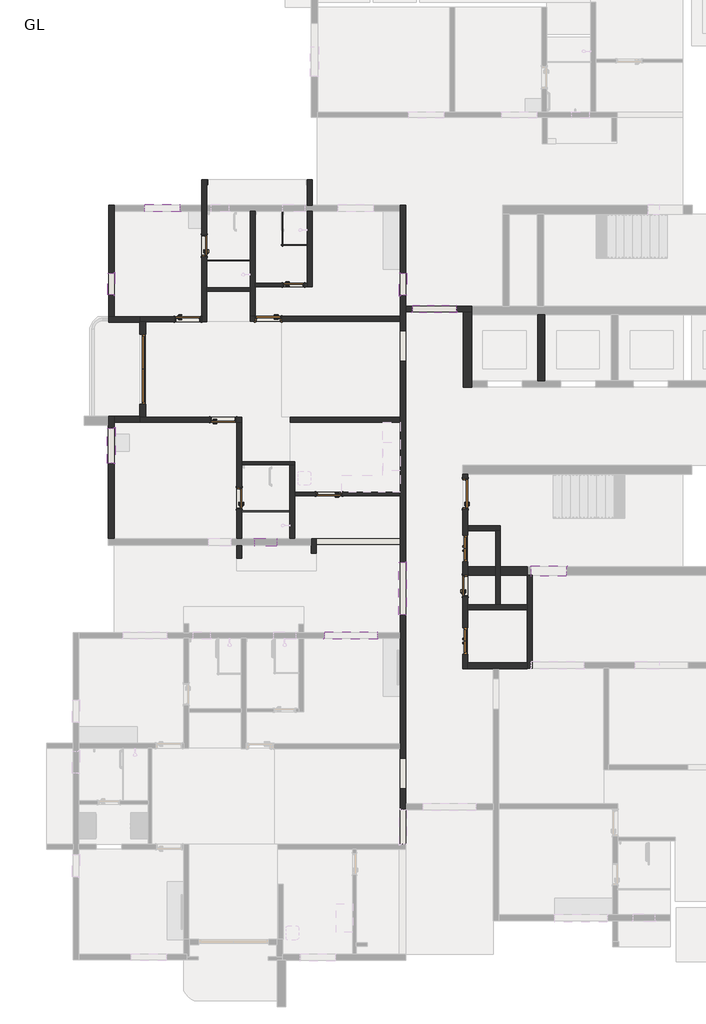
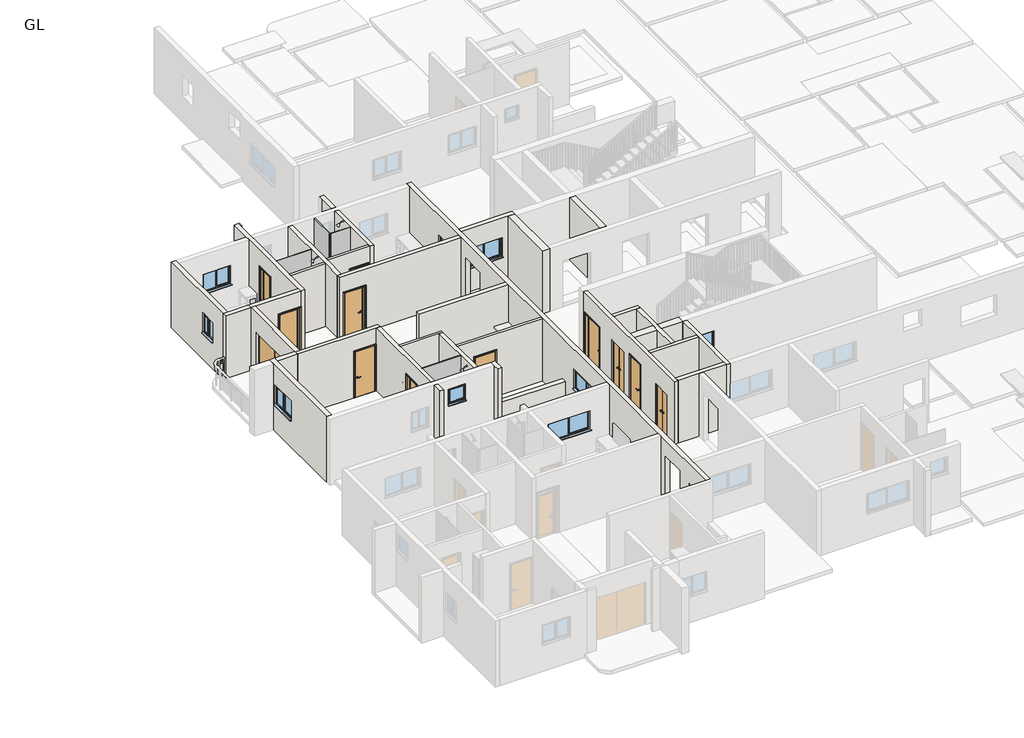
# One storey, part 2 of 14: 32 walls, 12 doors, 9 windows, 4 plates.
"""IFC4 building model written with IfcOpenShell, lengths in millimetres."""

from ifc_helpers import new_model, si_unit, frame, origin, origin_with_axes, place, context, project, spatial, polyline, outline, extrude, faceted_brep, transform, mapped, element, save
from components import doors_concept_extdbl_8_c180431f, doors_extdbl_flush_3_6b548a76, doors_intsgl_2_5_door_21b53886, doors_intsgl_2_5_door_57e365e7, doors_intsgl_2_5_door_fd097d29, doors_intsgl_2_5_door_b929695a, doors_intsgl_3_door_8261d8fb, doors_intsgl_3_door_f61d7fb9, doors_intsgl_3_door_77e94e6e, doors_intsgl_3_door_2f660dd7, doors_intsgl_3_5_a4e1cc10, system_panel_glazed_00f127ae, system_panel_glazed_4e689a8f, system_panel_glazed_de536e8c, system_panel_glazed_7a5adaf1, windows_dbl_plain_2_5_52f1e8c5, windows_dbl_plain_4_e08ba9e4, windows_dbl_plain_4_905afcad, windows_dbl_plain_4_ad201dc9, windows_dbl_plain_5_c7724a63, windows_dbl_plain_6_decf5736, windows_sgl_plain_2_5_1233c963

model = new_model("IFC4")

# Units and contexts
model_context = context("Model", 3, world=origin())
ifc_project = project(units=[si_unit("LENGTHUNIT", "METRE", prefix="MILLI")], contexts=[model_context])

# Site, building, storey
site = spatial("IfcSite", under=ifc_project)
building = spatial("IfcBuilding", under=site)
storey = spatial("IfcBuildingStorey", under=building, Name="GL", Elevation=0.0)

# Doors
placement = place(None, origin())
doors_concept_extdbl_8_shape = doors_concept_extdbl_8_c180431f(model_context)
element("IfcDoor", 1, ObjectType="Doors_Concept_ExtDbl : 8'", at=placement, inside=storey, context=model_context, shape_type="MappedRepresentation", body=[
    mapped(doors_concept_extdbl_8_shape, transform((-14465.3631346, 76757.5607361, 0.0), x_axis=(0.0, -1.0, 0.0), y_axis=(1.0, 0.0, 0.0), z_axis=(0.0, 0.0, 1.0))),
])
doors_extdbl_flush_3_shape = doors_extdbl_flush_3_6b548a76(model_context)
element("IfcDoor", 2, ObjectType="Doors_ExtDbl_Flush : 3'", at=placement, inside=storey, context=model_context, shape_type="MappedRepresentation", body=[
    mapped(doors_extdbl_flush_3_shape, transform((-3221.1847841, 67274.0128421, 0.0), x_axis=(0.0, -1.0, 0.0), y_axis=(1.0, 0.0, 0.0), z_axis=(0.0, 0.0, 1.0))),
])
element("IfcDoor", 3, ObjectType="Doors_ExtDbl_Flush : 3'", at=placement, inside=storey, context=model_context, shape_type="MappedRepresentation", body=[
    mapped(doors_extdbl_flush_3_shape, transform((-3221.1847841, 70498.5428421, 0.0), x_axis=(0.0, -1.0, 0.0), y_axis=(1.0, 0.0, 0.0), z_axis=(0.0, 0.0, 1.0))),
])
doors_intsgl_2_5_door_shape = doors_intsgl_2_5_door_21b53886(model_context)
element("IfcDoor", 4, ObjectType="Doors_IntSgl : 2.5' DOOR", at=placement, inside=storey, context=model_context, shape_type="MappedRepresentation", body=[
    mapped(doors_intsgl_2_5_door_shape, transform((-9206.9991708, 79690.7146999, 149.9616), x_axis=(1.0, 0.0, 0.0), y_axis=(0.0, 1.0, 0.0), z_axis=(0.0, 0.0, 1.0))),
])
doors_intsgl_2_5_door_2_shape = doors_intsgl_2_5_door_57e365e7(model_context)
element("IfcDoor", 5, ObjectType="Doors_IntSgl : 2.5' DOOR", at=placement, inside=storey, context=model_context, shape_type="MappedRepresentation", body=[
    mapped(doors_intsgl_2_5_door_2_shape, transform((-11094.7831346, 72249.3527724, 149.9616), x_axis=(0.0, 1.0, 0.0), y_axis=(-1.0, 0.0, 0.0), z_axis=(0.0, 0.0, 1.0))),
])
doors_intsgl_2_5_door_3_shape = doors_intsgl_2_5_door_fd097d29(model_context)
element("IfcDoor", 6, ObjectType="Doors_IntSgl : 2.5' DOOR", at=placement, inside=storey, context=model_context, shape_type="MappedRepresentation", body=[
    mapped(doors_intsgl_2_5_door_3_shape, transform((-12321.0850072, 81060.5334496, 149.9616), x_axis=(0.0, 1.0, 0.0), y_axis=(-1.0, 0.0, 0.0), z_axis=(0.0, 0.0, 1.0))),
])
doors_intsgl_2_5_door_4_shape = doors_intsgl_2_5_door_b929695a(model_context)
element("IfcDoor", 7, ObjectType="Doors_IntSgl : 2.5' DOOR", at=placement, inside=storey, context=model_context, shape_type="MappedRepresentation", body=[
    mapped(doors_intsgl_2_5_door_4_shape, transform((-3221.1847841, 69198.0628421, 149.9616), x_axis=(0.0, 1.0, 0.0), y_axis=(-1.0, 0.0, 0.0), z_axis=(0.0, 0.0, 1.0))),
])
doors_intsgl_3_door_shape = doors_intsgl_3_door_8261d8fb(model_context)
element("IfcDoor", 8, ObjectType="Doors_IntSgl : 3' DOOR", at=placement, inside=storey, context=model_context, shape_type="MappedRepresentation", body=[
    mapped(doors_intsgl_3_door_shape, transform((-10090.2131346, 78505.8807724, 149.9616), x_axis=(-1.0, 0.0, 0.0), y_axis=(0.0, -1.0, 0.0), z_axis=(0.0, 0.0, 1.0))),
])
doors_intsgl_3_door_2_shape = doors_intsgl_3_door_f61d7fb9(model_context)
element("IfcDoor", 9, ObjectType="Doors_IntSgl : 3' DOOR", at=placement, inside=storey, context=model_context, shape_type="MappedRepresentation", body=[
    mapped(doors_intsgl_3_door_2_shape, transform((-12890.5530072, 78496.4066999, 149.9616), x_axis=(1.0, 0.0, 0.0), y_axis=(0.0, 1.0, 0.0), z_axis=(0.0, 0.0, 1.0))),
])
doors_intsgl_3_door_3_shape = doors_intsgl_3_door_77e94e6e(model_context)
element("IfcDoor", 10, ObjectType="Doors_IntSgl : 3' DOOR", at=placement, inside=storey, context=model_context, shape_type="MappedRepresentation", body=[
    mapped(doors_intsgl_3_door_3_shape, transform((-7969.3131346, 72401.7527724, 149.9616), x_axis=(-1.0, 0.0, 0.0), y_axis=(0.0, -1.0, 0.0), z_axis=(0.0, 0.0, 1.0))),
])
doors_intsgl_3_door_4_shape = doors_intsgl_3_door_2f660dd7(model_context)
element("IfcDoor", 11, ObjectType="Doors_IntSgl : 3' DOOR", at=placement, inside=storey, context=model_context, shape_type="MappedRepresentation", body=[
    mapped(doors_intsgl_3_door_4_shape, transform((-11661.2031346, 74991.2827724, 149.9616), x_axis=(1.0, 0.0, 0.0), y_axis=(0.0, 1.0, 0.0), z_axis=(0.0, 0.0, 1.0))),
])
doors_intsgl_3_5_shape = doors_intsgl_3_5_a4e1cc10(model_context)
element("IfcDoor", 12, ObjectType="Doors_IntSgl : 3.5'", at=placement, inside=storey, context=model_context, shape_type="MappedRepresentation", body=[
    mapped(doors_intsgl_3_5_shape, transform((-3221.1847841, 72409.8178911, 0.0), x_axis=(0.0, 1.0, 0.0), y_axis=(-1.0, 0.0, 0.0), z_axis=(0.0, 0.0, 1.0))),
])

# Plates
system_panel_glazed_shape = system_panel_glazed_00f127ae(model_context)
element("IfcPlate", 13, ObjectType="System Panel : Glazed", at=placement, inside=storey, context=model_context, shape_type="MappedRepresentation", body=[
    mapped(system_panel_glazed_shape, transform((-9632.2131346, 81643.1046999, 0.0), x_axis=(0.0, -1.0, 0.0), y_axis=(1.0, 0.0, 0.0), z_axis=(0.0, 0.0, 1.0))),
])
system_panel_glazed_2_shape = system_panel_glazed_4e689a8f(model_context)
element("IfcPlate", 14, ObjectType="System Panel : Glazed", at=placement, inside=storey, context=model_context, shape_type="MappedRepresentation", body=[
    mapped(system_panel_glazed_2_shape, transform((-10179.437141, 71760.4027724, 0.0), x_axis=(1.0, 0.0, 0.0), y_axis=(0.0, 1.0, 0.0), z_axis=(0.0, 0.0, 1.0))),
])
system_panel_glazed_3_shape = system_panel_glazed_de536e8c(model_context)
element("IfcPlate", 15, ObjectType="System Panel : Glazed", at=placement, inside=storey, context=model_context, shape_type="MappedRepresentation", body=[
    mapped(system_panel_glazed_3_shape, transform((-11477.6830709, 80509.8646999, 0.0), x_axis=(1.0, 0.0, 0.0), y_axis=(0.0, 1.0, 0.0), z_axis=(0.0, 0.0, 1.0))),
])
system_panel_glazed_4_shape = system_panel_glazed_7a5adaf1(model_context)
element("IfcPlate", 16, ObjectType="System Panel : Glazed", at=placement, inside=storey, context=model_context, shape_type="MappedRepresentation", body=[
    mapped(system_panel_glazed_4_shape, transform((-9178.3061527, 81046.2046999, 0.0), x_axis=(1.0, 0.0, 0.0), y_axis=(0.0, 1.0, 0.0), z_axis=(0.0, 0.0, 1.0))),
])

# Walls
element("IfcWall", 17, ObjectType="W2", at=placement, inside=storey, context=model_context, shape_type="SweptSolid", body=[
    extrude(outline(polyline([(-9328.2131346, 75074.8487724), (-5492.8131346, 75074.8487724), (-5492.8131346, 74901.1127724), (-9328.2131346, 74901.1127724), (-9328.2131346, 75074.8487724)])), origin_with_axes(), (0.0, 0.0, 1.0), 3000.0),
])
element("IfcWall", 18, ObjectType="W2", at=placement, inside=storey, context=model_context, shape_type="Brep", body=[
    faceted_brep([(-5492.8131346, 78592.7487724, 0.0), (-10547.4131346, 78592.7487724, 0.0), (-10721.1491346, 78592.7487724, 0.0), (-10721.1491346, 78592.7487724, 3000.0), (-10547.4131346, 78592.7487724, 3000.0), (-5492.8131346, 78592.7487724, 3000.0), (-10547.4131346, 78592.7487724, 2259.9616), (-10547.4131346, 78592.7487724, 149.9616), (-9633.0131346, 78592.7487724, 149.9616), (-9633.0131346, 78592.7487724, 2259.9616), (-10721.1491346, 78419.0127724, 0.0), (-5492.8131346, 78419.0127724, 0.0), (-5492.8131346, 78419.0127724, 3000.0), (-10721.1491346, 78419.0127724, 3000.0), (-10547.4131346, 78419.0127724, 149.9616), (-10547.4131346, 78419.0127724, 2259.9616), (-9633.0131346, 78419.0127724, 2259.9616), (-9633.0131346, 78419.0127724, 149.9616)], [[[0, 1, 2, 3, 4, 5], [6, 7, 8, 9]], [[10, 11, 12, 13], [14, 15, 16, 17]], [[2, 1, 0, 11, 10]], [[5, 4, 3, 13, 12]], [[0, 5, 12, 11]], [[3, 2, 10, 13]], [[14, 7, 6, 15]], [[15, 6, 9, 16]], [[16, 9, 8, 17]], [[7, 14, 17, 8]]]),
])
element("IfcWall", 19, ObjectType="W2", at=placement, inside=storey, context=model_context, shape_type="Brep", body=[
    faceted_brep([(-10547.4131346, 78592.7487724, 0.0), (-10547.4131346, 79633.5646999, 0.0), (-10547.4131346, 79747.8646999, 0.0), (-10547.4131346, 82265.0046999, 0.0), (-10547.4131346, 82265.0046999, 3000.0), (-10547.4131346, 79747.8646999, 3000.0), (-10547.4131346, 79633.5646999, 3000.0), (-10547.4131346, 78592.7487724, 3000.0), (-10547.4131346, 78592.7487724, 2110.0), (-10721.1491346, 78592.7487724, 0.0), (-10721.1491346, 78592.7487724, 3000.0), (-10721.1491346, 79473.0334496, 3000.0), (-10721.1491346, 79587.3334496, 3000.0), (-10721.1491346, 82265.0046999, 3000.0), (-10721.1491346, 82265.0046999, 0.0), (-10721.1491346, 79587.3334496, 0.0), (-10721.1491346, 79473.0334496, 0.0)], [[[0, 1, 2, 3, 4, 5, 6, 7, 8]], [[9, 10, 11, 12, 13, 14, 15, 16]], [[3, 2, 1, 0, 9, 16, 15, 14]], [[7, 6, 5, 4, 13, 12, 11, 10]], [[0, 8, 7, 10, 9]], [[4, 3, 14, 13]]]),
])
element("IfcWall", 20, ObjectType="W2", at=placement, inside=storey, context=model_context, shape_type="Brep", body=[
    faceted_brep([(-12234.2170072, 78409.5386999, 0.0), (-12234.2170072, 79473.0334496, 0.0), (-12234.2170072, 79587.3334496, 0.0), (-12234.2170072, 82265.0046999, 0.0), (-12234.2170072, 82463.1246999, 0.0), (-12234.2170072, 83194.026856, 0.0), (-12234.2170072, 83367.762856, 0.0), (-12234.2170072, 83367.762856, 3000.0), (-12234.2170072, 83194.026856, 3000.0), (-12234.2170072, 82463.1246999, 3000.0), (-12234.2170072, 82265.0046999, 3000.0), (-12234.2170072, 79587.3334496, 3000.0), (-12234.2170072, 79473.0334496, 3000.0), (-12234.2170072, 78409.5386999, 3000.0), (-12234.2170072, 81441.5334496, 2259.9616), (-12234.2170072, 81441.5334496, 149.9616), (-12234.2170072, 80679.5334496, 149.9616), (-12234.2170072, 80679.5334496, 2259.9616), (-12407.9530072, 83367.762856, 0.0), (-12407.9530072, 82463.1246999, 0.0), (-12407.9530072, 82265.0046999, 0.0), (-12407.9530072, 78583.2746999, 0.0), (-12407.9530072, 78409.5386999, 0.0), (-12407.9530072, 78409.5386999, 3000.0), (-12407.9530072, 78583.2746999, 3000.0), (-12407.9530072, 82265.0046999, 3000.0), (-12407.9530072, 82463.1246999, 3000.0), (-12407.9530072, 83367.762856, 3000.0), (-12407.9530072, 81441.5334496, 149.9616), (-12407.9530072, 81441.5334496, 2259.9616), (-12407.9530072, 80679.5334496, 2259.9616), (-12407.9530072, 80679.5334496, 149.9616)], [[[0, 1, 2, 3, 4, 5, 6, 7, 8, 9, 10, 11, 12, 13], [14, 15, 16, 17]], [[18, 19, 20, 21, 22, 23, 24, 25, 26, 27], [28, 29, 30, 31]], [[6, 5, 4, 3, 2, 1, 0, 22, 21, 20, 19, 18]], [[13, 12, 11, 10, 9, 8, 7, 27, 26, 25, 24, 23]], [[0, 13, 23, 22]], [[7, 6, 18, 27]], [[28, 15, 14, 29]], [[29, 14, 17, 30]], [[30, 17, 16, 31]], [[15, 28, 31, 16]]]),
])
element("IfcWall", 21, ObjectType="W2", at=placement, inside=storey, context=model_context, shape_type="Brep", body=[
    faceted_brep([(-12407.9530072, 78583.2746999, 0.0), (-14564.4231346, 78583.2746999, 0.0), (-14564.4231346, 78583.2746999, 3000.0), (-12407.9530072, 78583.2746999, 3000.0), (-12433.3530072, 78583.2746999, 149.9616), (-12433.3530072, 78583.2746999, 2259.9616), (-13347.7530072, 78583.2746999, 2259.9616), (-13347.7530072, 78583.2746999, 149.9616), (-14564.4231346, 78409.5386999, 0.0), (-14366.3031346, 78409.5386999, 0.0), (-12407.9530072, 78409.5386999, 0.0), (-12407.9530072, 78409.5386999, 3000.0), (-14366.3031346, 78409.5386999, 3000.0), (-14564.4231346, 78409.5386999, 3000.0), (-12433.3530072, 78409.5386999, 2259.9616), (-12433.3530072, 78409.5386999, 149.9616), (-13347.7530072, 78409.5386999, 149.9616), (-13347.7530072, 78409.5386999, 2259.9616)], [[[0, 1, 2, 3], [4, 5, 6, 7]], [[8, 9, 10, 11, 12, 13], [14, 15, 16, 17]], [[1, 0, 10, 9, 8]], [[3, 2, 13, 12, 11]], [[0, 3, 11, 10]], [[2, 1, 8, 13]], [[4, 15, 14, 5]], [[5, 14, 17, 6]], [[6, 17, 16, 7]], [[15, 4, 7, 16]]]),
])
element("IfcWall", 22, ObjectType="W2", at=placement, inside=storey, context=model_context, shape_type="Brep", body=[
    faceted_brep([(-9336.8491346, 73417.7527724, 0.0), (-9336.8491346, 70838.3827724, 0.0), (-9336.8491346, 70838.3827724, 3000.0), (-9336.8491346, 73417.7527724, 3000.0), (-9163.1131346, 73417.7527724, 0.0), (-9163.1131346, 73417.7527724, 3000.0), (-9163.1131346, 72458.9027724, 3000.0), (-9163.1131346, 72344.6027724, 3000.0), (-9163.1131346, 70838.3827724, 3000.0), (-9163.1131346, 70838.3827724, 0.0), (-9163.1131346, 72344.6027724, 0.0), (-9163.1131346, 72458.9027724, 0.0)], [[[0, 1, 2, 3]], [[4, 5, 6, 7, 8, 9, 10, 11]], [[1, 0, 4, 11, 10, 9]], [[3, 2, 8, 7, 6, 5]], [[0, 3, 5, 4]], [[2, 1, 9, 8]]]),
])
element("IfcWall", 23, ObjectType="W2", at=placement, inside=storey, context=model_context, shape_type="Brep", body=[
    faceted_brep([(-8724.3991708, 83367.762856, 3000.0), (-8724.3991708, 83367.762856, 0.0), (-8724.3991708, 83194.026856, 0.0), (-8724.3991708, 82463.1246999, 0.0), (-8724.3991708, 82463.1246999, 3000.0), (-8724.3991708, 83194.026856, 3000.0), (-8550.6631708, 83367.762856, 0.0), (-8550.6631708, 83367.762856, 3000.0), (-8550.6631708, 82463.1246999, 3000.0), (-8550.6631708, 82463.1246999, 0.0)], [[[0, 1, 2, 3, 4, 5]], [[6, 7, 8, 9]], [[1, 6, 9, 3, 2]], [[7, 0, 5, 4, 8]], [[4, 3, 9, 8]], [[1, 0, 7, 6]]]),
    faceted_brep([(-8724.3991708, 79633.5646999, 0.0), (-8724.3991708, 79633.5646999, 3000.0), (-8724.3991708, 79747.8646999, 3000.0), (-8724.3991708, 82265.0046999, 3000.0), (-8724.3991708, 82265.0046999, 0.0), (-8724.3991708, 79747.8646999, 0.0), (-8550.6631708, 79633.5646999, 3000.0), (-8550.6631708, 79633.5646999, 0.0), (-8550.6631708, 82265.0046999, 0.0), (-8550.6631708, 82265.0046999, 3000.0)], [[[0, 1, 2, 3, 4, 5]], [[6, 7, 8, 9]], [[7, 0, 5, 4, 8]], [[1, 6, 9, 3, 2]], [[4, 3, 9, 8]], [[1, 0, 7, 6]]]),
])
element("IfcWall", 24, ObjectType="W2", at=placement, inside=storey, context=model_context, shape_type="SweptSolid", body=[
    extrude(outline(polyline([(-12234.2170072, 83367.762856), (-12196.1170072, 83367.762856), (-12196.1170072, 83194.026856), (-12234.2170072, 83194.026856), (-12234.2170072, 83367.762856)])), origin_with_axes(), (0.0, 0.0, 1.0), 3000.0),
])
element("IfcWall", 25, ObjectType="W2", at=placement, inside=storey, context=model_context, shape_type="Brep", body=[
    faceted_brep([(-8587.5491346, 70838.3827724, 3000.0), (-8587.5491346, 70838.3827724, 0.0), (-8587.5491346, 70609.7827724, 0.0), (-8587.5491346, 70335.4627724, 0.0), (-8587.5491346, 70335.4627724, 3000.0), (-8587.5491346, 70609.7827724, 3000.0), (-8413.8131346, 70838.3827724, 0.0), (-8413.8131346, 70838.3827724, 1171.2), (-8413.8131346, 70838.3827724, 3000.0), (-8413.8131346, 70335.4627724, 3000.0), (-8413.8131346, 70335.4627724, 0.0), (-8413.8131346, 70640.2627724, 0.0)], [[[0, 1, 2, 3, 4, 5]], [[6, 7, 8, 9, 10, 11]], [[3, 2, 1, 6, 11, 10]], [[4, 3, 10, 9]], [[0, 5, 4, 9, 8]], [[0, 8, 7, 6, 1]]]),
])
element("IfcWall", 26, ObjectType="W3", at=placement, inside=storey, context=model_context, shape_type="Brep", body=[
    faceted_brep([(-11010.9631346, 73417.7527724, 0.0), (-9336.8491346, 73417.7527724, 0.0), (-9163.1131346, 73417.7527724, 0.0), (-9163.1131346, 73417.7527724, 3000.0), (-9336.8491346, 73417.7527724, 3000.0), (-11010.9631346, 73417.7527724, 3000.0), (-11010.9631346, 73532.0527724, 0.0), (-11010.9631346, 73532.0527724, 3000.0), (-9163.1131346, 73532.0527724, 3000.0), (-9163.1131346, 73532.0527724, 0.0)], [[[0, 1, 2, 3, 4, 5]], [[6, 7, 8, 9]], [[2, 1, 0, 6, 9]], [[5, 4, 3, 8, 7]], [[0, 5, 7, 6]], [[3, 2, 9, 8]]]),
])
element("IfcWall", 27, ObjectType="W3", at=placement, inside=storey, context=model_context, shape_type="SweptSolid", body=[
    extrude(outline(polyline([(0.0, -9163.1131346), (0.0, -5492.8131346), (3000.0, -5492.8131346), (3000.0, -9163.1131346), (0.0, -9163.1131346)]), holes=[polyline([(149.9616, -8426.5131346), (2259.9616, -8426.5131346), (2259.9616, -7512.1131346), (149.9616, -7512.1131346), (149.9616, -8426.5131346)])]), frame((0.0, 72344.6027724, 0.0), z_axis=(0.0, 1.0, 0.0), x_axis=(0.0, 0.0, 1.0)), (0.0, 0.0, 1.0), 114.3),
])
element("IfcWall", 28, ObjectType="W3", at=placement, inside=storey, context=model_context, shape_type="SweptSolid", body=[
    extrude(outline(polyline([(-10721.1491346, 79473.0334496), (-12234.2170072, 79473.0334496), (-12234.2170072, 79587.3334496), (-10721.1491346, 79587.3334496), (-10721.1491346, 79473.0334496)])), origin_with_axes(), (0.0, 0.0, 1.0), 3000.0),
])
element("IfcWall", 29, ObjectType="W3", at=placement, inside=storey, context=model_context, shape_type="SweptSolid", body=[
    extrude(outline(polyline([(0.0, -10547.4131346), (0.0, -8724.3991708), (3000.0, -8724.3991708), (3000.0, -10547.4131346), (0.0, -10547.4131346)]), holes=[polyline([(2259.9616, -8825.9991708), (149.9616, -8825.9991708), (149.9616, -9587.9991708), (2259.9616, -9587.9991708), (2259.9616, -8825.9991708)])]), frame((0.0, 79633.5646999, 0.0), z_axis=(0.0, 1.0, 0.0), x_axis=(0.0, 0.0, 1.0)), (0.0, 0.0, 1.0), 114.3),
])
element("IfcWall", 30, ObjectType="W4", at=placement, inside=storey, context=model_context, shape_type="Brep", body=[
    faceted_brep([(-3288.0931346, 78750.2287724, 0.0), (-3288.0931346, 76131.4887724, 0.0), (-3288.0931346, 76131.4887724, 3000.0), (-3288.0931346, 78750.2287724, 3000.0), (-2983.2931346, 78750.2287724, 0.0), (-2983.2931346, 78750.2287724, 3000.0), (-2983.2931346, 78643.5487724, 3000.0), (-2983.2931346, 76353.9927724, 3000.0), (-2983.2931346, 76131.4887724, 3000.0), (-2983.2931346, 76131.4887724, 0.0), (-2983.2931346, 76353.9927724, 0.0), (-2983.2931346, 78643.5487724, 0.0)], [[[0, 1, 2, 3]], [[4, 5, 6, 7, 8, 9, 10, 11]], [[1, 0, 4, 11, 10, 9]], [[3, 2, 8, 7, 6, 5]], [[0, 3, 5, 4]], [[2, 1, 9, 8]]]),
])
element("IfcWall", 31, ObjectType="W4", at=placement, inside=storey, context=model_context, shape_type="Brep", body=[
    faceted_brep([(-1053.026306, 69566.3628421, 0.0), (-1053.026306, 69566.3628421, 3000.0), (-1988.0147841, 69566.3628421, 3000.0), (-1988.0147841, 69566.3628421, 0.0), (-1053.026306, 69871.1628421, 3000.0), (-1053.026306, 69871.1628421, 0.0), (-1988.0147841, 69871.1628421, 0.0), (-1988.0147841, 69871.1628421, 3000.0), (-1053.026306, 69866.1033979, 0.0), (-1053.026306, 69866.1033979, 3000.0)], [[[0, 1, 2, 3]], [[4, 5, 6, 7]], [[5, 8, 0, 3, 6]], [[1, 9, 4, 7, 2]], [[1, 0, 8, 5, 4, 9]], [[3, 2, 7, 6]]]),
    faceted_brep([(-3137.3647841, 69566.3628421, 3000.0), (-3137.3647841, 69566.3628421, 0.0), (-2155.6547841, 69566.3628421, 0.0), (-2155.6547841, 69566.3628421, 3000.0), (-3137.3647841, 69871.1628421, 0.0), (-3137.3647841, 69871.1628421, 3000.0), (-2155.6547841, 69871.1628421, 3000.0), (-2155.6547841, 69871.1628421, 0.0)], [[[0, 1, 2, 3]], [[4, 5, 6, 7]], [[1, 4, 7, 2]], [[5, 0, 3, 6]], [[1, 0, 5, 4]], [[3, 2, 7, 6]]]),
])
element("IfcWall", 32, ObjectType="W6", at=placement, inside=storey, context=model_context, shape_type="SweptSolid", body=[
    extrude(outline(polyline([(-686.4678446, 76353.9927724), (-686.4678446, 78643.5487724), (-442.6278446, 78643.5487724), (-442.6278446, 76353.9927724), (-686.4678446, 76353.9927724)])), origin_with_axes(), (0.0, 0.0, 1.0), 3000.0),
])
element("IfcWall", 33, ObjectType="W8", at=placement, inside=storey, context=model_context, shape_type="Brep", body=[
    faceted_brep([(-15452.1531346, 70838.3827724, 0.0), (-15452.1531346, 75105.5827724, 0.0), (-15452.1531346, 75105.5827724, 3000.0), (-15452.1531346, 70838.3827724, 3000.0), (-15452.1531346, 73479.9827724, 2110.0), (-15452.1531346, 74699.1827724, 2110.0), (-15452.1531346, 74699.1827724, 1200.0), (-15452.1531346, 73479.9827724, 1200.0), (-15665.5131346, 70838.3827724, 0.0), (-15665.5131346, 70838.3827724, 3000.0), (-15665.5131346, 74800.7827724, 3000.0), (-15665.5131346, 75105.5827724, 3000.0), (-15665.5131346, 75105.5827724, 0.0), (-15665.5131346, 74800.7827724, 0.0), (-15665.5131346, 73479.9827724, 2110.0), (-15665.5131346, 73479.9827724, 1200.0), (-15665.5131346, 74699.1827724, 1200.0), (-15665.5131346, 74699.1827724, 2110.0)], [[[0, 1, 2, 3], [4, 5, 6, 7]], [[8, 9, 10, 11, 12, 13], [14, 15, 16, 17]], [[1, 0, 8, 13, 12]], [[3, 2, 11, 10, 9]], [[0, 3, 9, 8]], [[2, 1, 12, 11]], [[15, 14, 4, 7]], [[16, 15, 7, 6]], [[17, 16, 6, 5]], [[14, 17, 5, 4]]]),
])
element("IfcWall", 34, ObjectType="W9", at=placement, inside=storey, context=model_context, shape_type="Brep", body=[
    faceted_brep([(-14564.4231346, 74907.4627724, 0.0), (-11178.6031346, 74907.4627724, 0.0), (-11010.9631346, 74907.4627724, 0.0), (-11010.9631346, 74907.4627724, 3000.0), (-11178.6031346, 74907.4627724, 3000.0), (-14564.4231346, 74907.4627724, 3000.0), (-11204.0031346, 74907.4627724, 2259.9616), (-11204.0031346, 74907.4627724, 149.9616), (-12118.4031346, 74907.4627724, 149.9616), (-12118.4031346, 74907.4627724, 2259.9616), (-11010.9631346, 75075.1027724, 0.0), (-14366.3031346, 75075.1027724, 0.0), (-14564.4231346, 75075.1027724, 0.0), (-14564.4231346, 75075.1027724, 3000.0), (-14366.3031346, 75075.1027724, 3000.0), (-11010.9631346, 75075.1027724, 3000.0), (-11204.0031346, 75075.1027724, 149.9616), (-11204.0031346, 75075.1027724, 2259.9616), (-12118.4031346, 75075.1027724, 2259.9616), (-12118.4031346, 75075.1027724, 149.9616)], [[[0, 1, 2, 3, 4, 5], [6, 7, 8, 9]], [[10, 11, 12, 13, 14, 15], [16, 17, 18, 19]], [[2, 1, 0, 12, 11, 10]], [[5, 4, 3, 15, 14, 13]], [[3, 2, 10, 15]], [[0, 5, 13, 12]], [[16, 7, 6, 17]], [[17, 6, 9, 18]], [[18, 9, 8, 19]], [[7, 16, 19, 8]]]),
])
element("IfcWall", 35, ObjectType="W9", at=placement, inside=storey, context=model_context, shape_type="Brep", body=[
    faceted_brep([(-11178.6031346, 70160.2027724, 0.0), (-11178.6031346, 70160.2027724, 3000.0), (-11178.6031346, 70609.7827724, 3000.0), (-11178.6031346, 70609.7827724, 0.0), (-11010.9631346, 70160.2027724, 3000.0), (-11010.9631346, 70160.2027724, 0.0), (-11010.9631346, 70609.7827724, 0.0), (-11010.9631346, 70609.7827724, 3000.0)], [[[0, 1, 2, 3]], [[4, 5, 6, 7]], [[5, 0, 3, 6]], [[1, 0, 5, 4]], [[1, 4, 7, 2]], [[3, 2, 7, 6]]]),
    faceted_brep([(-11178.6031346, 74907.4627724, 3000.0), (-11178.6031346, 74907.4627724, 0.0), (-11178.6031346, 70838.3827724, 0.0), (-11178.6031346, 70838.3827724, 3000.0), (-11178.6031346, 72630.3527724, 149.9616), (-11178.6031346, 72630.3527724, 2259.9616), (-11178.6031346, 71868.3527724, 2259.9616), (-11178.6031346, 71868.3527724, 149.9616), (-11010.9631346, 74907.4627724, 0.0), (-11010.9631346, 74907.4627724, 3000.0), (-11010.9631346, 73532.0527724, 3000.0), (-11010.9631346, 73417.7527724, 3000.0), (-11010.9631346, 70838.3827724, 3000.0), (-11010.9631346, 70838.3827724, 0.0), (-11010.9631346, 73417.7527724, 0.0), (-11010.9631346, 73532.0527724, 0.0), (-11010.9631346, 72630.3527724, 2259.9616), (-11010.9631346, 72630.3527724, 149.9616), (-11010.9631346, 71868.3527724, 149.9616), (-11010.9631346, 71868.3527724, 2259.9616)], [[[0, 1, 2, 3], [4, 5, 6, 7]], [[8, 9, 10, 11, 12, 13, 14, 15], [16, 17, 18, 19]], [[1, 8, 15, 14, 13, 2]], [[9, 0, 3, 12, 11, 10]], [[1, 0, 9, 8]], [[3, 2, 13, 12]], [[4, 17, 16, 5]], [[5, 16, 19, 6]], [[18, 7, 6, 19]], [[17, 4, 7, 18]]]),
])
element("IfcWall", 36, ObjectType="W9", at=placement, inside=storey, context=model_context, shape_type="Brep", body=[
    faceted_brep([(-3305.0047841, 66313.8928421, 3000.0), (-3305.0047841, 73095.6178911, 3000.0), (-3305.0047841, 73095.6178911, 0.0), (-3305.0047841, 72943.2178911, 0.0), (-3305.0047841, 72943.2178911, 2110.0), (-3305.0047841, 71876.4178911, 2110.0), (-3305.0047841, 71876.4178911, 0.0), (-3305.0047841, 70955.7428421, 0.0), (-3305.0047841, 70955.7428421, 2110.0), (-3305.0047841, 70041.3428421, 2110.0), (-3305.0047841, 70041.3428421, 0.0), (-3305.0047841, 67731.2128421, 0.0), (-3305.0047841, 67731.2128421, 2110.0), (-3305.0047841, 66816.8128421, 2110.0), (-3305.0047841, 66816.8128421, 0.0), (-3305.0047841, 66313.8928421, 0.0), (-3305.0047841, 69579.0628421, 149.9616), (-3305.0047841, 69579.0628421, 2259.9616), (-3305.0047841, 68817.0628421, 2259.9616), (-3305.0047841, 68817.0628421, 149.9616), (-3137.3647841, 73095.6178911, 3000.0), (-3137.3647841, 71293.5628421, 3000.0), (-3137.3647841, 71125.9228421, 3000.0), (-3137.3647841, 69871.1628421, 3000.0), (-3137.3647841, 69566.3628421, 3000.0), (-3137.3647841, 68537.6628421, 3000.0), (-3137.3647841, 68370.0228421, 3000.0), (-3137.3647841, 66512.0128421, 3000.0), (-3137.3647841, 66313.8928421, 3000.0), (-3137.3647841, 66313.8928421, 0.0), (-3137.3647841, 66512.0128421, 0.0), (-3137.3647841, 66816.8128421, 0.0), (-3137.3647841, 66816.8128421, 2110.0), (-3137.3647841, 67731.2128421, 2110.0), (-3137.3647841, 67731.2128421, 0.0), (-3137.3647841, 68370.0228421, 0.0), (-3137.3647841, 68537.6628421, 0.0), (-3137.3647841, 69566.3628421, 0.0), (-3137.3647841, 69871.1628421, 0.0), (-3137.3647841, 70041.3428421, 0.0), (-3137.3647841, 70041.3428421, 2110.0), (-3137.3647841, 70955.7428421, 2110.0), (-3137.3647841, 70955.7428421, 0.0), (-3137.3647841, 71125.9228421, 0.0), (-3137.3647841, 71293.5628421, 0.0), (-3137.3647841, 71876.4178911, 0.0), (-3137.3647841, 71876.4178911, 2110.0), (-3137.3647841, 72943.2178911, 2110.0), (-3137.3647841, 72943.2178911, 0.0), (-3137.3647841, 73095.6178911, 0.0), (-3137.3647841, 69579.0628421, 2259.9616), (-3137.3647841, 69579.0628421, 149.9616), (-3137.3647841, 68817.0628421, 149.9616), (-3137.3647841, 68817.0628421, 2259.9616)], [[[0, 1, 2, 3, 4, 5, 6, 7, 8, 9, 10, 11, 12, 13, 14, 15], [16, 17, 18, 19]], [[20, 21, 22, 23, 24, 25, 26, 27, 28, 29, 30, 31, 32, 33, 34, 35, 36, 37, 38, 39, 40, 41, 42, 43, 44, 45, 46, 47, 48, 49], [50, 51, 52, 53]], [[29, 15, 14, 31, 30]], [[2, 49, 48, 3]], [[6, 45, 44, 43, 42, 7]], [[34, 11, 10, 39, 38, 37, 36, 35]], [[1, 0, 28, 27, 26, 25, 24, 23, 22, 21, 20]], [[0, 15, 29, 28]], [[2, 1, 20, 49]], [[47, 4, 3, 48]], [[4, 47, 46, 5]], [[5, 46, 45, 6]], [[34, 33, 12, 11]], [[32, 31, 14, 13]], [[33, 32, 13, 12]], [[42, 41, 8, 7]], [[40, 39, 10, 9]], [[41, 40, 9, 8]], [[16, 51, 50, 17]], [[17, 50, 53, 18]], [[18, 53, 52, 19]], [[51, 16, 19, 52]]]),
])
element("IfcWall", 37, ObjectType="W9", at=placement, inside=storey, context=model_context, shape_type="Brep", body=[
    faceted_brep([(-3137.3647841, 71125.9228421, 0.0), (-2155.6547841, 71125.9228421, 0.0), (-1988.0147841, 71125.9228421, 0.0), (-1988.0147841, 71125.9228421, 3000.0), (-2155.6547841, 71125.9228421, 3000.0), (-3137.3647841, 71125.9228421, 3000.0), (-3137.3647841, 71293.5628421, 0.0), (-3137.3647841, 71293.5628421, 3000.0), (-1988.0147841, 71293.5628421, 3000.0), (-1988.0147841, 71293.5628421, 0.0)], [[[0, 1, 2, 3, 4, 5]], [[6, 7, 8, 9]], [[2, 1, 0, 6, 9]], [[5, 4, 3, 8, 7]], [[0, 5, 7, 6]], [[3, 2, 9, 8]]]),
])
element("IfcWall", 38, ObjectType="W9", at=placement, inside=storey, context=model_context, shape_type="Brep", body=[
    faceted_brep([(-2155.6547841, 71125.9228421, 0.0), (-2155.6547841, 69871.1628421, 0.0), (-2155.6547841, 69566.3628421, 0.0), (-2155.6547841, 68537.6628421, 0.0), (-2155.6547841, 68537.6628421, 3000.0), (-2155.6547841, 69566.3628421, 3000.0), (-2155.6547841, 69871.1628421, 3000.0), (-2155.6547841, 71125.9228421, 3000.0), (-1988.0147841, 71125.9228421, 0.0), (-1988.0147841, 71125.9228421, 3000.0), (-1988.0147841, 69871.1628421, 3000.0), (-1988.0147841, 69566.3628421, 3000.0), (-1988.0147841, 68537.6628421, 3000.0), (-1988.0147841, 68537.6628421, 0.0), (-1988.0147841, 69566.3628421, 0.0), (-1988.0147841, 69871.1628421, 0.0)], [[[0, 1, 2, 3, 4, 5, 6, 7]], [[8, 9, 10, 11, 12, 13, 14, 15]], [[3, 2, 1, 0, 8, 15, 14, 13]], [[7, 6, 5, 4, 12, 11, 10, 9]], [[0, 7, 9, 8]], [[4, 3, 13, 12]]]),
])
element("IfcWall", 39, ObjectType="W9", at=placement, inside=storey, context=model_context, shape_type="Brep", body=[
    faceted_brep([(-3137.3647841, 68370.0228421, 0.0), (-1053.026306, 68370.0228421, 0.0), (-1053.026306, 68370.0228421, 3000.0), (-3137.3647841, 68370.0228421, 3000.0), (-3137.3647841, 68537.6628421, 0.0), (-3137.3647841, 68537.6628421, 3000.0), (-2155.6547841, 68537.6628421, 3000.0), (-1988.0147841, 68537.6628421, 3000.0), (-1053.026306, 68537.6628421, 3000.0), (-1053.026306, 68537.6628421, 0.0), (-1988.0147841, 68537.6628421, 0.0), (-2155.6547841, 68537.6628421, 0.0)], [[[0, 1, 2, 3]], [[4, 5, 6, 7, 8, 9, 10, 11]], [[1, 0, 4, 11, 10, 9]], [[3, 2, 8, 7, 6, 5]], [[0, 3, 5, 4]], [[2, 1, 9, 8]]]),
])
element("IfcWall", 40, ObjectType="W9", at=placement, inside=storey, context=model_context, shape_type="Brep", body=[
    faceted_brep([(-1053.026306, 69561.3033979, 0.0), (-1053.026306, 68537.6628421, 0.0), (-1053.026306, 68370.0228421, 0.0), (-1053.026306, 66512.0128421, 0.0), (-1053.026306, 66317.7028421, 0.0), (-1053.026306, 66317.7028421, 3000.0), (-1053.026306, 66512.0128421, 3000.0), (-1053.026306, 68370.0228421, 3000.0), (-1053.026306, 68537.6628421, 3000.0), (-1053.026306, 69561.3033979, 3000.0), (-885.386306, 66317.7028421, 0.0), (-885.386306, 66531.0628421, 0.0), (-885.386306, 69561.3033979, 0.0), (-885.386306, 69561.3033979, 3000.0), (-885.386306, 66531.0628421, 3000.0), (-885.386306, 66317.7028421, 3000.0), (-885.386306, 66317.7028421, 2110.0), (-885.386306, 66531.0628421, 2110.0), (-885.386306, 66531.0628421, 1200.0), (-885.386306, 66317.7028421, 1200.0), (-910.786306, 66317.7028421, 1200.0), (-910.786306, 66317.7028421, 2110.0), (-910.786306, 66531.0628421, 2110.0), (-910.786306, 66531.0628421, 1200.0)], [[[0, 1, 2, 3, 4, 5, 6, 7, 8, 9]], [[10, 11, 12, 13, 14, 15, 16, 17, 18, 19]], [[4, 3, 2, 1, 0, 12, 11, 10]], [[9, 8, 7, 6, 5, 15, 14, 13]], [[0, 9, 13, 12]], [[5, 4, 10, 19, 20, 21, 16, 15]], [[22, 23, 18, 17]], [[23, 22, 21, 20]], [[23, 20, 19, 18]], [[21, 22, 17, 16]]]),
])
element("IfcWall", 41, ObjectType="WALL 1", at=placement, inside=storey, context=model_context, shape_type="Brep", body=[
    faceted_brep([(-5492.8131346, 61396.9487724, 2110.0), (-5492.8131346, 60177.7487724, 2110.0), (-5492.8131346, 60177.7487724, 3000.0), (-5492.8131346, 63521.9127724, 3000.0), (-5492.8131346, 63695.6487724, 3000.0), (-5492.8131346, 67367.4734152, 3000.0), (-5492.8131346, 67565.5934152, 3000.0), (-5492.8131346, 72344.6027724, 3000.0), (-5492.8131346, 72458.9027724, 3000.0), (-5492.8131346, 74901.1127724, 3000.0), (-5492.8131346, 75074.8487724, 3000.0), (-5492.8131346, 78419.0127724, 3000.0), (-5492.8131346, 78592.7487724, 3000.0), (-5492.8131346, 82265.0046999, 3000.0), (-5492.8131346, 82463.1246999, 3000.0), (-5492.8131346, 82470.3127724, 3000.0), (-5492.8131346, 82470.3127724, 0.0), (-5492.8131346, 82463.1246999, 0.0), (-5492.8131346, 82265.0046999, 0.0), (-5492.8131346, 78592.7487724, 0.0), (-5492.8131346, 78419.0127724, 0.0), (-5492.8131346, 75074.8487724, 0.0), (-5492.8131346, 74901.1127724, 0.0), (-5492.8131346, 72458.9027724, 0.0), (-5492.8131346, 72344.6027724, 0.0), (-5492.8131346, 70838.3827724, 0.0), (-5492.8131346, 70640.2627724, 0.0), (-5492.8131346, 67565.5934152, 0.0), (-5492.8131346, 67367.4734152, 0.0), (-5492.8131346, 63695.6487724, 0.0), (-5492.8131346, 63521.9127724, 0.0), (-5492.8131346, 60177.7487724, 0.0), (-5492.8131346, 60177.7487724, 1200.0), (-5492.8131346, 61396.9487724, 1200.0), (-5492.8131346, 62124.9127724, 2259.9616), (-5492.8131346, 62124.9127724, 149.9616), (-5492.8131346, 63191.7127724, 149.9616), (-5492.8131346, 63191.7127724, 2259.9616), (-5492.8131346, 68188.5280938, 2110.0), (-5492.8131346, 68188.5280938, 1200.0), (-5492.8131346, 70017.3280938, 1200.0), (-5492.8131346, 70017.3280938, 2110.0), (-5492.8131346, 80091.3487724, 2110.0), (-5492.8131346, 79329.3487724, 2110.0), (-5492.8131346, 79329.3487724, 1200.0), (-5492.8131346, 80091.3487724, 1200.0), (-5492.8131346, 77022.0127724, 2259.9616), (-5492.8131346, 77022.0127724, 149.9616), (-5492.8131346, 78088.8127724, 149.9616), (-5492.8131346, 78088.8127724, 2259.9616), (-5294.6931346, 60177.7487724, 3000.0), (-5294.6931346, 60177.7487724, 2110.0), (-5294.6931346, 61396.9487724, 2110.0), (-5294.6931346, 61396.9487724, 1200.0), (-5294.6931346, 60177.7487724, 1200.0), (-5294.6931346, 60177.7487724, 0.0), (-5294.6931346, 61393.3927724, 0.0), (-5294.6931346, 61591.5127724, 0.0), (-5294.6931346, 78750.2287724, 0.0), (-5294.6931346, 78948.3487724, 0.0), (-5294.6931346, 82470.3127724, 0.0), (-5294.6931346, 82470.3127724, 3000.0), (-5294.6931346, 78948.3487724, 3000.0), (-5294.6931346, 78750.2287724, 3000.0), (-5294.6931346, 61591.5127724, 3000.0), (-5294.6931346, 61393.3927724, 3000.0), (-5294.6931346, 62124.9127724, 2259.9616), (-5294.6931346, 63191.7127724, 2259.9616), (-5294.6931346, 63191.7127724, 149.9616), (-5294.6931346, 62124.9127724, 149.9616), (-5294.6931346, 68188.5280938, 2110.0), (-5294.6931346, 70017.3280938, 2110.0), (-5294.6931346, 70017.3280938, 1200.0), (-5294.6931346, 68188.5280938, 1200.0), (-5294.6931346, 80091.3487724, 2110.0), (-5294.6931346, 80091.3487724, 1200.0), (-5294.6931346, 79329.3487724, 1200.0), (-5294.6931346, 79329.3487724, 2110.0), (-5294.6931346, 77022.0127724, 2259.9616), (-5294.6931346, 78088.8127724, 2259.9616), (-5294.6931346, 78088.8127724, 149.9616), (-5294.6931346, 77022.0127724, 149.9616)], [[[0, 1, 2, 3, 4, 5, 6, 7, 8, 9, 10, 11, 12, 13, 14, 15, 16, 17, 18, 19, 20, 21, 22, 23, 24, 25, 26, 27, 28, 29, 30, 31, 32, 33], [34, 35, 36, 37], [38, 39, 40, 41], [42, 43, 44, 45], [46, 47, 48, 49]], [[50, 51, 52, 53, 54, 55, 56, 57, 58, 59, 60, 61, 62, 63, 64, 65], [66, 67, 68, 69], [70, 71, 72, 73], [74, 75, 76, 77], [78, 79, 80, 81]], [[31, 30, 29, 28, 27, 26, 25, 24, 23, 22, 21, 20, 19, 18, 17, 16, 60, 59, 58, 57, 56, 55]], [[15, 14, 13, 12, 11, 10, 9, 8, 7, 6, 5, 4, 3, 2, 50, 65, 64, 63, 62, 61]], [[16, 15, 61, 60]], [[53, 52, 0, 33]], [[54, 53, 33, 32]], [[52, 51, 1, 0]], [[35, 34, 66, 69]], [[36, 35, 69, 68]], [[37, 36, 68, 67]], [[34, 37, 67, 66]], [[32, 31, 55, 54]], [[2, 1, 51, 50]], [[39, 38, 70, 73]], [[40, 39, 73, 72]], [[41, 40, 72, 71]], [[38, 41, 71, 70]], [[75, 74, 42, 45]], [[76, 75, 45, 44]], [[77, 76, 44, 43]], [[74, 77, 43, 42]], [[47, 46, 78, 81]], [[48, 47, 81, 80]], [[49, 48, 80, 79]], [[46, 49, 79, 78]]]),
])
element("IfcWall", 42, ObjectType="WALL 1", at=placement, inside=storey, context=model_context, shape_type="Brep", body=[
    faceted_brep([(-5294.6931346, 78750.2287724, 0.0), (-3288.0931346, 78750.2287724, 0.0), (-2983.2931346, 78750.2287724, 0.0), (-2983.2931346, 78750.2287724, 3000.0), (-3288.0931346, 78750.2287724, 3000.0), (-5294.6931346, 78750.2287724, 3000.0), (-5053.3931346, 78750.2287724, 2110.0), (-3529.3931346, 78750.2287724, 2110.0), (-3529.3931346, 78750.2287724, 1200.0), (-5053.3931346, 78750.2287724, 1200.0), (-5294.6931346, 78948.3487724, 0.0), (-5294.6931346, 78948.3487724, 3000.0), (-2983.2931346, 78948.3487724, 3000.0), (-2983.2931346, 78948.3487724, 0.0), (-5053.3931346, 78948.3487724, 2110.0), (-5053.3931346, 78948.3487724, 1200.0), (-3529.3931346, 78948.3487724, 1200.0), (-3529.3931346, 78948.3487724, 2110.0)], [[[0, 1, 2, 3, 4, 5], [6, 7, 8, 9]], [[10, 11, 12, 13], [14, 15, 16, 17]], [[2, 1, 0, 10, 13]], [[5, 4, 3, 12, 11]], [[0, 5, 11, 10]], [[3, 2, 13, 12]], [[15, 14, 6, 9]], [[16, 15, 9, 8]], [[17, 16, 8, 7]], [[14, 17, 7, 6]]]),
])
element("IfcWall", 43, ObjectType="WALL 1", at=placement, inside=storey, context=model_context, shape_type="SweptSolid", body=[
    extrude(outline(polyline([(-8413.8131346, 70838.3827724), (-5492.8131346, 70838.3827724), (-5492.8131346, 70640.2627724), (-8413.8131346, 70640.2627724), (-8413.8131346, 70838.3827724)])), origin_with_axes(), (0.0, 0.0, 1.0), 1171.2),
])
element("IfcWall", 44, ObjectType="WALL 1", at=placement, inside=storey, context=model_context, shape_type="Brep", body=[
    faceted_brep([(-15445.8031346, 74907.4627724, 0.0), (-14564.4231346, 74907.4627724, 0.0), (-14564.4231346, 74907.4627724, 3000.0), (-15445.8031346, 74907.4627724, 3000.0), (-15445.8031346, 75105.5827724, 0.0), (-15445.8031346, 75105.5827724, 3000.0), (-14564.4231346, 75105.5827724, 3000.0), (-14564.4231346, 75105.5827724, 0.0), (-14564.4231346, 75075.1027724, 0.0), (-14564.4231346, 75075.1027724, 3000.0)], [[[0, 1, 2, 3]], [[4, 5, 6, 7]], [[1, 0, 4, 7, 8]], [[3, 2, 9, 6, 5]], [[0, 3, 5, 4]], [[2, 1, 8, 7, 6, 9]]]),
])
element("IfcWall", 45, ObjectType="WALL 1", at=placement, inside=storey, context=model_context, shape_type="Brep", body=[
    faceted_brep([(-14366.3031346, 75075.1027724, 0.0), (-14366.3031346, 75538.3607361, 0.0), (-14366.3031346, 75538.3607361, 2110.0), (-14366.3031346, 77976.7607361, 2110.0), (-14366.3031346, 77976.7607361, 0.0), (-14366.3031346, 78409.5386999, 0.0), (-14366.3031346, 78409.5386999, 3000.0), (-14366.3031346, 75075.1027724, 3000.0), (-14564.4231346, 75538.3607361, 2110.0), (-14564.4231346, 75538.3607361, 0.0), (-14564.4231346, 75105.5827724, 0.0), (-14564.4231346, 75075.1027724, 0.0), (-14564.4231346, 75075.1027724, 3000.0), (-14564.4231346, 75105.5827724, 3000.0), (-14564.4231346, 78385.1546999, 3000.0), (-14564.4231346, 78409.5386999, 3000.0), (-14564.4231346, 78409.5386999, 0.0), (-14564.4231346, 78385.1546999, 0.0), (-14564.4231346, 77976.7607361, 0.0), (-14564.4231346, 77976.7607361, 2110.0)], [[[0, 1, 2, 3, 4, 5, 6, 7]], [[8, 9, 10, 11, 12, 13, 14, 15, 16, 17, 18, 19]], [[11, 10, 9, 1, 0]], [[18, 17, 16, 5, 4]], [[7, 6, 15, 14, 13, 12]], [[6, 5, 16, 15]], [[0, 7, 12, 11]], [[4, 3, 19, 18]], [[2, 1, 9, 8]], [[3, 2, 8, 19]]]),
])
element("IfcWall", 46, ObjectType="WALL 1", at=placement, inside=storey, context=model_context, shape_type="Brep", body=[
    faceted_brep([(-14564.4231346, 78583.2746999, 0.0), (-15458.5031346, 78583.2746999, 0.0), (-15656.6231346, 78583.2746999, 0.0), (-15656.6231346, 78583.2746999, 3000.0), (-15458.5031346, 78583.2746999, 3000.0), (-14564.4231346, 78583.2746999, 3000.0), (-14564.4231346, 78385.1546999, 0.0), (-14564.4231346, 78385.1546999, 3000.0), (-15656.6231346, 78385.1546999, 3000.0), (-15656.6231346, 78385.1546999, 0.0), (-14564.4231346, 78409.5386999, 0.0), (-14564.4231346, 78409.5386999, 3000.0)], [[[0, 1, 2, 3, 4, 5]], [[6, 7, 8, 9]], [[2, 1, 0, 10, 6, 9]], [[5, 4, 3, 8, 7, 11]], [[0, 5, 11, 7, 6, 10]], [[3, 2, 9, 8]]]),
])
element("IfcWall", 47, ObjectType="WALL 1", at=placement, inside=storey, context=model_context, shape_type="Brep", body=[
    faceted_brep([(-15458.5031346, 78583.2746999, 0.0), (-15458.5031346, 82265.0046999, 0.0), (-15458.5031346, 82463.1246999, 0.0), (-15458.5031346, 82463.1246999, 3000.0), (-15458.5031346, 82265.0046999, 3000.0), (-15458.5031346, 78583.2746999, 3000.0), (-15458.5031346, 79345.2746999, 2110.0), (-15458.5031346, 80107.2746999, 2110.0), (-15458.5031346, 80107.2746999, 1200.0), (-15458.5031346, 79345.2746999, 1200.0), (-15656.6231346, 78583.2746999, 0.0), (-15656.6231346, 78583.2746999, 3000.0), (-15656.6231346, 82463.1246999, 3000.0), (-15656.6231346, 82463.1246999, 0.0), (-15656.6231346, 79345.2746999, 2110.0), (-15656.6231346, 79345.2746999, 1200.0), (-15656.6231346, 80107.2746999, 1200.0), (-15656.6231346, 80107.2746999, 2110.0)], [[[0, 1, 2, 3, 4, 5], [6, 7, 8, 9]], [[10, 11, 12, 13], [14, 15, 16, 17]], [[2, 1, 0, 10, 13]], [[5, 4, 3, 12, 11]], [[0, 5, 11, 10]], [[3, 2, 13, 12]], [[15, 14, 6, 9]], [[16, 15, 9, 8]], [[17, 16, 8, 7]], [[14, 17, 7, 6]]]),
])
element("IfcWall", 48, ObjectType="WALL 1", at=placement, inside=storey, context=model_context, shape_type="Brep", body=[
    faceted_brep([(-3137.3647841, 66313.8928421, 0.0), (-2242.4865436, 66313.8928421, 0.0), (-2044.3665436, 66313.8928421, 0.0), (-1053.026306, 66313.8928421, 0.0), (-1053.026306, 66313.8928421, 3000.0), (-2044.3665436, 66313.8928421, 3000.0), (-2242.4865436, 66313.8928421, 3000.0), (-3137.3647841, 66313.8928421, 3000.0), (-3137.3647841, 66512.0128421, 0.0), (-3137.3647841, 66512.0128421, 3000.0), (-1053.026306, 66512.0128421, 3000.0), (-1053.026306, 66512.0128421, 0.0), (-1053.026306, 66317.7028421, 0.0), (-1053.026306, 66317.7028421, 3000.0)], [[[0, 1, 2, 3, 4, 5, 6, 7]], [[8, 9, 10, 11]], [[3, 2, 1, 0, 8, 11, 12]], [[7, 6, 5, 4, 13, 10, 9]], [[0, 7, 9, 8]], [[4, 3, 12, 11, 10, 13]]]),
])

# Windows
windows_dbl_plain_2_5_shape = windows_dbl_plain_2_5_52f1e8c5(model_context)
element("IfcWindow", 49, ObjectType="Windows_Dbl_Plain : 2.5'", at=placement, inside=storey, context=model_context, shape_type="MappedRepresentation", body=[
    mapped(windows_dbl_plain_2_5_shape, transform((-15549.1065668, 80011.2746999, 0.0), x_axis=(0.0, 1.0, 0.0), y_axis=(-1.0, 0.0, 0.0), z_axis=(0.0, 0.0, 1.0))),
])
element("IfcWindow", 50, ObjectType="Windows_Dbl_Plain : 2.5'", at=placement, inside=storey, context=model_context, shape_type="MappedRepresentation", body=[
    mapped(windows_dbl_plain_2_5_shape, transform((-5402.2097024, 79425.3487724, 0.0), x_axis=(0.0, -1.0, 0.0), y_axis=(1.0, 0.0, 0.0), z_axis=(0.0, 0.0, 1.0))),
])
windows_dbl_plain_4_shape = windows_dbl_plain_4_e08ba9e4(model_context)
element("IfcWindow", 51, ObjectType="Windows_Dbl_Plain : 4'", at=placement, inside=storey, context=model_context, shape_type="MappedRepresentation", body=[
    mapped(windows_dbl_plain_4_shape, transform((-13497.1031346, 82355.6081321, 0.0), x_axis=(1.0, 0.0, 0.0), y_axis=(0.0, 1.0, 0.0), z_axis=(0.0, 0.0, 1.0))),
])
windows_dbl_plain_4_2_shape = windows_dbl_plain_4_905afcad(model_context)
element("IfcWindow", 52, ObjectType="Windows_Dbl_Plain : 4'", at=placement, inside=storey, context=model_context, shape_type="MappedRepresentation", body=[
    mapped(windows_dbl_plain_4_2_shape, transform((-15550.3765668, 74374.5827724, 0.0), x_axis=(0.0, 1.0, 0.0), y_axis=(-1.0, 0.0, 0.0), z_axis=(0.0, 0.0, 1.0))),
])
windows_dbl_plain_4_3_shape = windows_dbl_plain_4_ad201dc9(model_context)
element("IfcWindow", 53, ObjectType="Windows_Dbl_Plain : 4'", at=placement, inside=storey, context=model_context, shape_type="MappedRepresentation", body=[
    mapped(windows_dbl_plain_4_3_shape, transform((-586.186306, 69722.1599657, 0.0), x_axis=(-1.0, 0.0, 0.0), y_axis=(0.0, -1.0, 0.0), z_axis=(0.0, 0.0, 1.0))),
])
windows_dbl_plain_5_shape = windows_dbl_plain_5_c7724a63(model_context)
element("IfcWindow", 54, ObjectType="Windows_Dbl_Plain : 5'", at=placement, inside=storey, context=model_context, shape_type="MappedRepresentation", body=[
    mapped(windows_dbl_plain_5_shape, transform((-4006.3931346, 78840.8322045, 0.0), x_axis=(1.0, 0.0, 0.0), y_axis=(0.0, 1.0, 0.0), z_axis=(0.0, 0.0, 1.0))),
])
windows_dbl_plain_6_shape = windows_dbl_plain_6_decf5736(model_context)
element("IfcWindow", 55, ObjectType="Windows_Dbl_Plain : 6'", at=placement, inside=storey, context=model_context, shape_type="MappedRepresentation", body=[
    mapped(windows_dbl_plain_6_shape, transform((-6921.9146601, 67458.0768474, 0.0), x_axis=(1.0, 0.0, 0.0), y_axis=(0.0, 1.0, 0.0), z_axis=(0.0, 0.0, 1.0))),
])
element("IfcWindow", 56, ObjectType="Windows_Dbl_Plain : 6'", at=placement, inside=storey, context=model_context, shape_type="MappedRepresentation", body=[
    mapped(windows_dbl_plain_6_shape, transform((-5385.2965668, 69387.9280938, 0.0), x_axis=(0.0, 1.0, 0.0), y_axis=(-1.0, 0.0, 0.0), z_axis=(0.0, 0.0, 1.0))),
])
windows_sgl_plain_2_5_shape = windows_sgl_plain_2_5_1233c963(model_context)
element("IfcWindow", 57, ObjectType="Windows_Sgl_Plain : 2.5'", at=placement, inside=storey, context=model_context, shape_type="MappedRepresentation", body=[
    mapped(windows_sgl_plain_2_5_shape, transform((-10175.0491346, 70732.5393402, 480.8), x_axis=(-1.0, 0.0, 0.0), y_axis=(0.0, -1.0, 0.0), z_axis=(0.0, 0.0, 1.0))),
])

save(model, "model.ifc")

# Revit data of these elements
# Type "Doors_Concept_ExtDbl : 8'"
#   Type Mark = "53"
#   Type Comments = "External Double"
#   Operation = "DoubleDoorSingleSwing"
#   Construction Type Id = "GSP4R"
#   Keynote = "L10"
#   Analytic Construction = "1/8 in Pilkington single glazing"
#   Visual Light Transmittance = 0.9
#   Thickness = 0.144357 ft
#   Solar Heat Gain Coefficient = 0.78
#   Rough Width = 8.0 ft
#   Rough Height = 6.922572 ft
#   Heat Transfer Coefficient (U) = 3.6886 W/(m²·K)
#   FrameWidth = 0.137795 ft
#   FrameOffset - External = 0.082021 ft
#   Height = 6.922572 ft
#   Width = 8.0 ft
#   Define Thermal Properties by = 1
#   Function = 1
#   Material Door = Door - Glazing
#   Material Frame = Concept
#   Wall Closure = (empty or 0)
# Type "Doors_ExtDbl_Flush : 3'"
#   Type Mark = "55"
#   Type Comments = "External Double"
#   Operation = "DoubleDoorSingleSwing"
#   Keynote = "L20"
#   Analytic Construction = "Metal"
#   Wrap Layers (Ext) from Ext = 0.336286 ft
#   Wrap Layers (Int) from Ext = 0.582349 ft
#   Thickness = 0.144357 ft
#   Rough Width = 3.0 ft
#   Rough Height = 6.922572 ft
#   O/A Frame Width = 0.209974 ft
#   Heat Transfer Coefficient (U) = 3.7021 W/(m²·K)
#   Handle Z Distance = 3.444882 ft
#   FrameWidth = 0.137795 ft
#   FrameOffset - External = 0.082021 ft
#   FrameDepth = 0.291995 ft
#   Door Panel Width = 1.326115 ft
#   Door Panel Thickness = 0.144357 ft
#   Door Panel Height = 6.56168 ft
#   Cill Thickness = 0.178806 ft
#   Cill Projection = 0.098425 ft
#   Handle X Distance = 0.246063 ft
#   Height = 6.922572 ft
#   Structural Tolerance = 0.021325 ft
#   Tolerance = 0.009843 ft
#   Undercut = 0.013123 ft
#   Width = 3.0 ft
#   Cill Extension = 0.082021 ft
#   Cavity Closer Width = 0.164042 ft
#   Cavity Closer Offset from Ext = 0.336286 ft
#   Cavity Closer Depth = 0.278871 ft
#   Vis - Ironmongery = yes
#   Vis - Cavity Closers = yes
#   Function = 1
#   Material Door = Door - Panel
#   Material Frame = Door - Frame/Mullion
#   Material Ironmongery = Door - Handle
#   Visual Light Transmittance = 0
#   Thermal Resistance (R) = 0
#   Solar Heat Gain Coefficient = 0
#   Wall Closure = (empty or 0)
# Type "Doors_IntSgl : 2.5' DOOR"
#   Type Mark = "47"
#   Type Comments = "Internal Single"
#   Operation = "SingleSwingRight"
#   Manufacturer = "Revit"
#   Keynote = "L20"
#   Description = "Internal Single Door"
#   Analytic Construction = "Metal"
#   UnderCut = 0.026247 ft
#   Tolerance = 0.006562 ft
#   Thickness = 0.124672 ft
#   Thermal Resistance (R) = 0.270117 (m²·K)/W
#   Structural Tolerance = 0.026247 ft
#   StopDepth = 0.104987 ft
#   Stop Thickness = 0.062336 ft
#   Rough Width = 2.5 ft
#   Rough Height = 6.922572 ft
#   Height to Top Lock Rail = 3.28084 ft
#   Heat Transfer Coefficient (U) = 3.7021 W/(m²·K)
#   Handle Z Distance = 2.952756 ft
#   Handle X Distance = 0.246063 ft
#   Frame Thickness = 0.104987 ft
#   Door Panel Width = 2.224409 ft
#   Door Panel Thickness = 0.124672 ft
#   Door Panel Offset = 0.0 ft
#   Height = 6.922572 ft
#   Width = 2.5 ft
#   Door Panel Height = 6.75853 ft
#   Architrave Setback = 0.016404 ft
#   Vis - Ironmongery = yes
#   Material Ironmongery = Door - Handle
#   Material Frame = Door - Frame/Mullion (1)
#   Material Door = Door - Panel
#   Material Architrave = Door - Architrave
#   Visual Light Transmittance = 0
#   Solar Heat Gain Coefficient = 0
#   Function = (empty or 0)
#   Wall Closure = (empty or 0)
# Type "Doors_IntSgl : 3' DOOR"
#   Type Mark = "46"
#   Type Comments = "Internal Single"
#   Operation = "SingleSwingRight"
#   Manufacturer = "Revit"
#   Keynote = "L20"
#   Description = "Internal Single Door"
#   Analytic Construction = "Metal"
#   UnderCut = 0.026247 ft
#   Tolerance = 0.006562 ft
#   Thickness = 0.124672 ft
#   Thermal Resistance (R) = 0.270117 (m²·K)/W
#   Structural Tolerance = 0.026247 ft
#   StopDepth = 0.104987 ft
#   Stop Thickness = 0.062336 ft
#   Rough Width = 3.0 ft
#   Rough Height = 6.922572 ft
#   Height to Top Lock Rail = 3.28084 ft
#   Heat Transfer Coefficient (U) = 3.7021 W/(m²·K)
#   Handle Z Distance = 2.952756 ft
#   Handle X Distance = 0.246063 ft
#   Frame Thickness = 0.104987 ft
#   Door Panel Width = 2.724409 ft
#   Door Panel Thickness = 0.124672 ft
#   Door Panel Offset = 0.0 ft
#   Height = 6.922572 ft
#   Width = 3.0 ft
#   Door Panel Height = 6.75853 ft
#   Architrave Setback = 0.016404 ft
#   Vis - Ironmongery = yes
#   Material Ironmongery = Door - Handle
#   Material Frame = Door - Frame/Mullion (1)
#   Material Door = Door - Panel
#   Material Architrave = Door - Architrave
#   Visual Light Transmittance = 0
#   Solar Heat Gain Coefficient = 0
#   Function = (empty or 0)
#   Wall Closure = (empty or 0)
# Type "Doors_IntSgl : 3.5'"
#   Type Mark = "51"
#   Type Comments = "Internal Single"
#   Operation = "SingleSwingRight"
#   Manufacturer = "Revit"
#   Keynote = "L20"
#   Description = "Internal Single Door"
#   Analytic Construction = "Metal"
#   UnderCut = 0.026247 ft
#   Tolerance = 0.006562 ft
#   Thickness = 0.124672 ft
#   Thermal Resistance (R) = 0.270117 (m²·K)/W
#   Structural Tolerance = 0.026247 ft
#   StopDepth = 0.104987 ft
#   Stop Thickness = 0.062336 ft
#   Rough Width = 3.5 ft
#   Rough Height = 6.922572 ft
#   Height to Top Lock Rail = 3.28084 ft
#   Heat Transfer Coefficient (U) = 3.7021 W/(m²·K)
#   Handle Z Distance = 2.952756 ft
#   Handle X Distance = 0.246063 ft
#   Frame Thickness = 0.104987 ft
#   Door Panel Width = 3.224409 ft
#   Door Panel Thickness = 0.124672 ft
#   Door Panel Offset = 0.0 ft
#   Height = 6.922572 ft
#   Width = 3.5 ft
#   Door Panel Height = 6.75853 ft
#   Architrave Setback = 0.016404 ft
#   Vis - Ironmongery = yes
#   Material Ironmongery = Door - Handle
#   Material Frame = Door - Frame/Mullion (1)
#   Material Door = Door - Panel
#   Material Architrave = Door - Architrave
#   Visual Light Transmittance = 0
#   Solar Heat Gain Coefficient = 0
#   Function = (empty or 0)
#   Wall Closure = (empty or 0)
# Type "System Panel : Glazed"
#   Keynote = "H11"
#   Construction Type Id = "GSP4R"
#   Analytic Construction = "1/8 in Pilkington single glazing"
#   Visual Light Transmittance = 0.9
#   Solar Heat Gain Coefficient = 0.86
#   Heat Transfer Coefficient (U) = 6.7069 W/(m²·K)
#   Define Thermal Properties by = 1
# Type "W2"
#   Keynote = "F10"
#   Layers, outside or top first: 0.57 ft "Brick, Common" (function 1)
# Type "W3"
#   Keynote = "F10"
#   Layers, outside or top first: 0.375 ft "Brick, Common" (function 1)
# Type "W4"
#   Keynote = "F10"
#   Layers, outside or top first: 1.0 ft "Brick, Common" (function 1)
# Type "W6"
#   Keynote = "F10"
#   Layers, outside or top first: 0.8 ft "Brick, Common" (function 1)
# Type "W8"
#   Keynote = "F10"
#   Layers, outside or top first: 0.7 ft "Brick, Common" (function 1)
# Type "W9"
#   Keynote = "F10"
#   Layers, outside or top first: 0.55 ft "Brick, Common" (function 1)
# Type "WALL 1"
#   Keynote = "F10"
#   Layers, outside or top first: 0.65 ft "Brick, Common" (function 1)
# Type "Windows_Dbl_Plain : 2.5'"
#   Type Mark = "57"
#   Operation = "DoublePanelVertical"
#   Construction Type Id = "GSP4R"
#   Manufacturer = "Revit"
#   Keynote = "L10"
